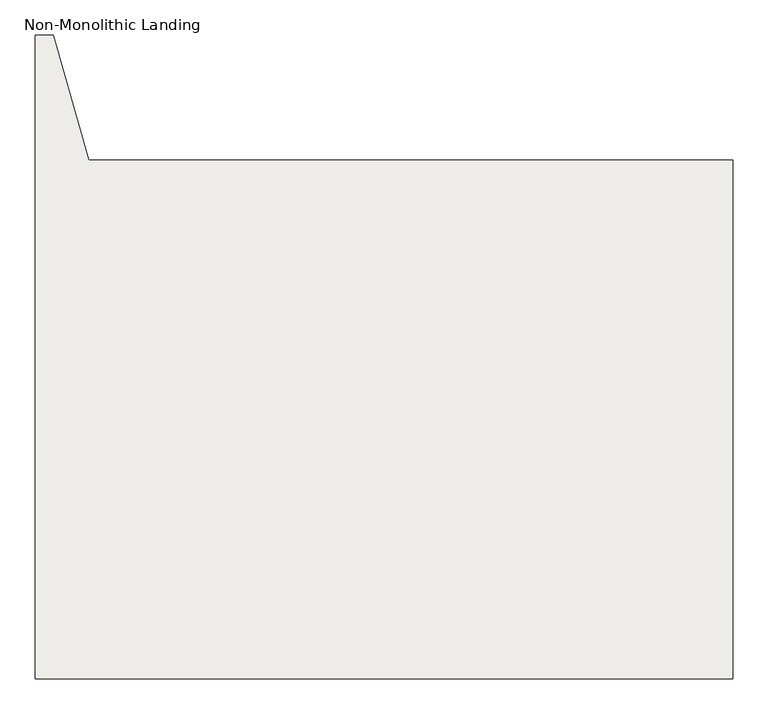
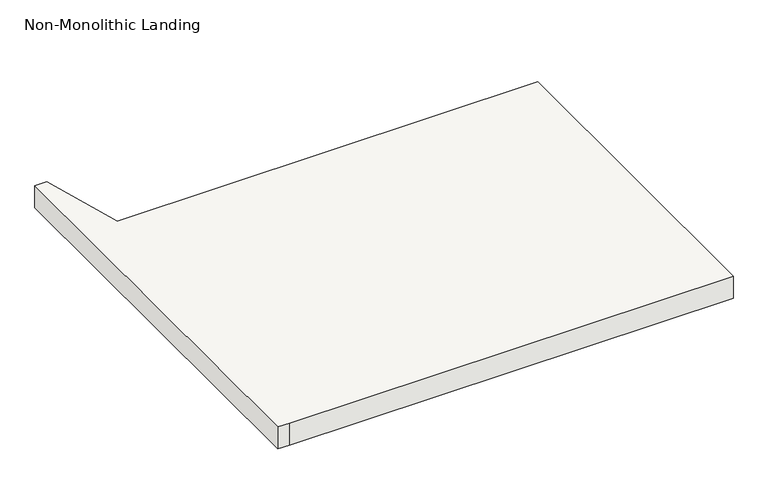
"""IFC4 building model written with IfcOpenShell, lengths in millimetres: slab geometry, Non-Monolithic Landing."""

from ifc_helpers import new_model, si_unit, origin, place, context, project, spatial, faceted_brep, source, transform, mapped, element, save


def non_monolithic_landing_1f105fa5(model_context):
    return source(origin(), model_context, "Body", "Brep", [
        faceted_brep([(-6768.1118598, 2384.3368529, 2370.6666667), (-6768.1118598, 2384.3368529, 2351.6166667), (-7682.5118598, 2384.3368529, 2351.6166667), (-7682.5118598, 2384.3368529, 2370.6666667), (-6768.1118598, 2358.9368529, 2326.2166667), (-7675.2547169, 2358.9368529, 2326.2166667), (-7733.3118598, 2562.1368529, 2370.6666667), (-7758.7118598, 2562.1368529, 2370.6666667), (-7758.7118598, 1647.7368529, 2370.6666667), (-7733.3118598, 1647.7368529, 2370.6666667), (-6768.1118598, 1647.7368529, 2370.6666667), (-7675.2547169, 2358.9368529, 2319.8666667), (-6768.1118598, 2358.9368529, 2319.8666667), (-6768.1118598, 1647.7368529, 2319.8666667), (-7733.3118598, 1647.7368529, 2319.8666667), (-7758.7118598, 1647.7368529, 2319.8666667), (-7758.7118598, 2562.1368529, 2319.8666667), (-7733.3118598, 2562.1368529, 2319.8666667)], [[[0, 1, 2, 3]], [[1, 4, 5, 2]], [[6, 7, 8, 9, 10, 0, 3]], [[11, 12, 13, 14, 15, 16, 17]], [[12, 11, 5, 4]], [[11, 17, 6, 3, 2, 5]], [[7, 6, 17, 16]], [[8, 7, 16, 15]], [[9, 8, 15, 14]], [[10, 9, 14, 13]], [[0, 10, 13, 12, 4, 1]]]),
    ])


if __name__ == "__main__":
    model = new_model("IFC4")
    model_context = context("Model", 3, world=origin())
    ifc_project = project(units=[si_unit("LENGTHUNIT", "METRE", prefix="MILLI")], contexts=[model_context])
    site = spatial("IfcSite", under=ifc_project)
    building = spatial("IfcBuilding", under=site)
    placement = place(None, origin())
    non_monolithic_landing_shape = non_monolithic_landing_1f105fa5(model_context)
    element("IfcSlab", 1, ObjectType="Non-Monolithic Landing", at=placement, inside=building, context=model_context, shape_type="MappedRepresentation", body=[
        mapped(non_monolithic_landing_shape, transform((0.0, 0.0, 0.0), x_axis=(1.0, 0.0, 0.0), y_axis=(0.0, 1.0, 0.0), z_axis=(0.0, 0.0, 1.0))),
    ])
    save(model, "model.ifc")
